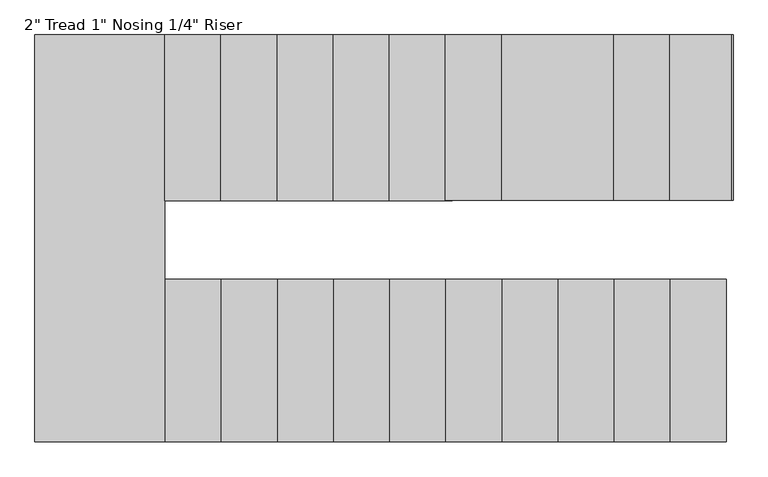
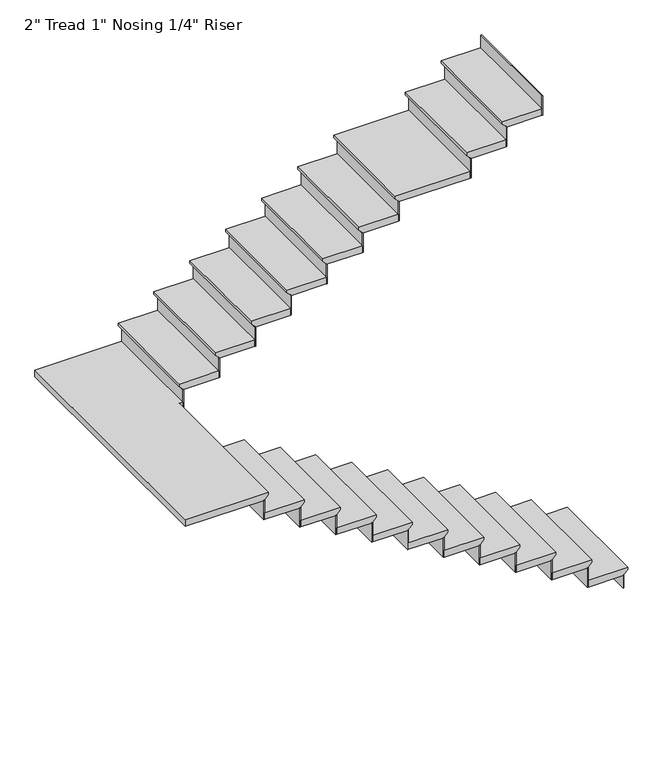
"""IFC4 building model written with IfcOpenShell, lengths in millimetres: stair flight geometry."""

from ifc_helpers import new_model, si_unit, origin, place, context, project, spatial, faceted_brep, source, transform, mapped, element, save


def stair_flight_d547b7c1(model_context):
    return source(origin(), model_context, "Body", "Brep", [
        faceted_brep([(-3117.2664982, -7431.6600272, 6222.0928571), (-3117.2664982, -7431.6600272, 6241.1428571), (-3117.2664982, -8168.2600272, 6241.1428571), (-3117.2664982, -8168.2600272, 6222.0928571), (-3142.6664982, -7431.6600272, 6196.6928571), (-3142.6664982, -8168.2600272, 6196.6928571), (-3396.6664982, -7431.6600272, 6241.1428571), (-3396.6664982, -8168.2600272, 6241.1428571), (-3142.6664982, -8168.2600272, 6190.3428571), (-3396.6664982, -8168.2600272, 6190.3428571), (-3396.6664982, -7431.6600272, 6190.3428571), (-3142.6664982, -7431.6600272, 6190.3428571)], [[[0, 1, 2, 3]], [[4, 0, 3, 5]], [[2, 1, 6, 7]], [[8, 9, 10, 11]], [[2, 7, 9, 8, 5, 3]], [[8, 11, 4, 5]], [[6, 1, 0, 4, 11, 10]], [[7, 6, 10, 9]]]),
        faceted_brep([(-3142.6664982, -7431.6600272, 6190.3428571), (-3142.6664982, -7431.6600272, 6096.0), (-3149.0164982, -7431.6600272, 6096.0), (-3149.0164982, -7431.6600272, 6190.3428571), (-3142.6664982, -8168.2600272, 6190.3428571), (-3149.0164982, -8168.2600272, 6190.3428571), (-3149.0164982, -8168.2600272, 6096.0), (-3142.6664982, -8168.2600272, 6096.0)], [[[0, 1, 2, 3]], [[4, 5, 6, 7]], [[1, 0, 4, 7]], [[2, 1, 7, 6]], [[3, 2, 6, 5]], [[0, 3, 5, 4]]]),
        faceted_brep([(-3396.6664982, -7431.6600272, 6335.4857143), (-3396.6664982, -7431.6600272, 6190.3428571), (-3403.0164982, -7431.6600272, 6190.3428571), (-3403.0164982, -7431.6600272, 6335.4857143), (-3396.6664982, -8168.2600272, 6335.4857143), (-3403.0164982, -8168.2600272, 6335.4857143), (-3403.0164982, -8168.2600272, 6190.3428571), (-3396.6664982, -8168.2600272, 6190.3428571)], [[[0, 1, 2, 3]], [[4, 5, 6, 7]], [[1, 0, 4, 7]], [[2, 1, 7, 6]], [[3, 2, 6, 5]], [[0, 3, 5, 4]]]),
        faceted_brep([(-3371.2664982, -8168.2600272, 6386.2857143), (-3371.2664982, -7431.6600272, 6386.2857143), (-3650.6664982, -7431.6600272, 6386.2857143), (-3650.6664982, -8168.2600272, 6386.2857143), (-3396.6664982, -8168.2600272, 6335.4857143), (-3650.6664982, -8168.2600272, 6335.4857143), (-3650.6664982, -7431.6600272, 6335.4857143), (-3396.6664982, -7431.6600272, 6335.4857143), (-3396.6664982, -8168.2600272, 6341.8357143), (-3371.2664982, -8168.2600272, 6367.2357143), (-3396.6664982, -7431.6600272, 6341.8357143), (-3371.2664982, -7431.6600272, 6367.2357143)], [[[0, 1, 2, 3]], [[4, 5, 6, 7]], [[0, 3, 5, 4, 8, 9]], [[4, 7, 10, 8]], [[2, 1, 11, 10, 7, 6]], [[3, 2, 6, 5]], [[11, 1, 0, 9]], [[10, 11, 9, 8]]]),
        faceted_brep([(-3650.6664982, -7431.6600272, 6480.6285714), (-3650.6664982, -7431.6600272, 6335.4857143), (-3657.0164982, -7431.6600272, 6335.4857143), (-3657.0164982, -7431.6600272, 6480.6285714), (-3650.6664982, -8168.2600272, 6480.6285714), (-3657.0164982, -8168.2600272, 6480.6285714), (-3657.0164982, -8168.2600272, 6335.4857143), (-3650.6664982, -8168.2600272, 6335.4857143)], [[[0, 1, 2, 3]], [[4, 5, 6, 7]], [[1, 0, 4, 7]], [[2, 1, 7, 6]], [[3, 2, 6, 5]], [[0, 3, 5, 4]]]),
        faceted_brep([(-3625.2664982, -8168.2600272, 6531.4285714), (-3625.2664982, -7431.6600272, 6531.4285714), (-3904.6664982, -7431.6600272, 6531.4285714), (-3904.6664982, -8168.2600272, 6531.4285714), (-3650.6664982, -8168.2600272, 6480.6285714), (-3904.6664982, -8168.2600272, 6480.6285714), (-3904.6664982, -7431.6600272, 6480.6285714), (-3650.6664982, -7431.6600272, 6480.6285714), (-3650.6664982, -8168.2600272, 6486.9785714), (-3625.2664982, -8168.2600272, 6512.3785714), (-3650.6664982, -7431.6600272, 6486.9785714), (-3625.2664982, -7431.6600272, 6512.3785714)], [[[0, 1, 2, 3]], [[4, 5, 6, 7]], [[0, 3, 5, 4, 8, 9]], [[4, 7, 10, 8]], [[2, 1, 11, 10, 7, 6]], [[3, 2, 6, 5]], [[11, 1, 0, 9]], [[10, 11, 9, 8]]]),
        faceted_brep([(-3904.6664982, -7431.6600272, 6625.7714286), (-3904.6664982, -7431.6600272, 6480.6285714), (-3911.0164982, -7431.6600272, 6480.6285714), (-3911.0164982, -7431.6600272, 6625.7714286), (-3904.6664982, -8168.2600272, 6625.7714286), (-3911.0164982, -8168.2600272, 6625.7714286), (-3911.0164982, -8168.2600272, 6480.6285714), (-3904.6664982, -8168.2600272, 6480.6285714)], [[[0, 1, 2, 3]], [[4, 5, 6, 7]], [[1, 0, 4, 7]], [[2, 1, 7, 6]], [[3, 2, 6, 5]], [[0, 3, 5, 4]]]),
        faceted_brep([(-3879.2664982, -8168.2600272, 6676.5714286), (-3879.2664982, -7431.6600272, 6676.5714286), (-4158.6664982, -7431.6600272, 6676.5714286), (-4158.6664982, -8168.2600272, 6676.5714286), (-3904.6664982, -8168.2600272, 6625.7714286), (-4158.6664982, -8168.2600272, 6625.7714286), (-4158.6664982, -7431.6600272, 6625.7714286), (-3904.6664982, -7431.6600272, 6625.7714286), (-3904.6664982, -8168.2600272, 6632.1214286), (-3879.2664982, -8168.2600272, 6657.5214286), (-3904.6664982, -7431.6600272, 6632.1214286), (-3879.2664982, -7431.6600272, 6657.5214286)], [[[0, 1, 2, 3]], [[4, 5, 6, 7]], [[0, 3, 5, 4, 8, 9]], [[4, 7, 10, 8]], [[2, 1, 11, 10, 7, 6]], [[3, 2, 6, 5]], [[11, 1, 0, 9]], [[10, 11, 9, 8]]]),
        faceted_brep([(-4158.6664982, -7431.6600272, 6770.9142857), (-4158.6664982, -7431.6600272, 6625.7714286), (-4165.0164982, -7431.6600272, 6625.7714286), (-4165.0164982, -7431.6600272, 6770.9142857), (-4158.6664982, -8168.2600272, 6770.9142857), (-4165.0164982, -8168.2600272, 6770.9142857), (-4165.0164982, -8168.2600272, 6625.7714286), (-4158.6664982, -8168.2600272, 6625.7714286)], [[[0, 1, 2, 3]], [[4, 5, 6, 7]], [[1, 0, 4, 7]], [[2, 1, 7, 6]], [[3, 2, 6, 5]], [[0, 3, 5, 4]]]),
        faceted_brep([(-4133.2664982, -8168.2600272, 6821.7142857), (-4133.2664982, -7431.6600272, 6821.7142857), (-4412.6664982, -7431.6600272, 6821.7142857), (-4412.6664982, -8168.2600272, 6821.7142857), (-4158.6664982, -8168.2600272, 6770.9142857), (-4412.6664982, -8168.2600272, 6770.9142857), (-4412.6664982, -7431.6600272, 6770.9142857), (-4158.6664982, -7431.6600272, 6770.9142857), (-4158.6664982, -8168.2600272, 6777.2642857), (-4133.2664982, -8168.2600272, 6802.6642857), (-4158.6664982, -7431.6600272, 6777.2642857), (-4133.2664982, -7431.6600272, 6802.6642857)], [[[0, 1, 2, 3]], [[4, 5, 6, 7]], [[0, 3, 5, 4, 8, 9]], [[4, 7, 10, 8]], [[2, 1, 11, 10, 7, 6]], [[3, 2, 6, 5]], [[11, 1, 0, 9]], [[10, 11, 9, 8]]]),
        faceted_brep([(-4412.6664982, -7431.6600272, 6916.0571429), (-4412.6664982, -7431.6600272, 6770.9142857), (-4419.0164982, -7431.6600272, 6770.9142857), (-4419.0164982, -7431.6600272, 6916.0571429), (-4412.6664982, -8168.2600272, 6916.0571429), (-4419.0164982, -8168.2600272, 6916.0571429), (-4419.0164982, -8168.2600272, 6770.9142857), (-4412.6664982, -8168.2600272, 6770.9142857)], [[[0, 1, 2, 3]], [[4, 5, 6, 7]], [[1, 0, 4, 7]], [[2, 1, 7, 6]], [[3, 2, 6, 5]], [[0, 3, 5, 4]]]),
        faceted_brep([(-4387.2664982, -8168.2600272, 6966.8571429), (-4387.2664982, -7431.6600272, 6966.8571429), (-4666.6664982, -7431.6600272, 6966.8571429), (-4666.6664982, -8168.2600272, 6966.8571429), (-4412.6664982, -8168.2600272, 6916.0571429), (-4666.6664982, -8168.2600272, 6916.0571429), (-4666.6664982, -7431.6600272, 6916.0571429), (-4412.6664982, -7431.6600272, 6916.0571429), (-4412.6664982, -8168.2600272, 6922.4071429), (-4387.2664982, -8168.2600272, 6947.8071429), (-4412.6664982, -7431.6600272, 6922.4071429), (-4387.2664982, -7431.6600272, 6947.8071429)], [[[0, 1, 2, 3]], [[4, 5, 6, 7]], [[0, 3, 5, 4, 8, 9]], [[4, 7, 10, 8]], [[2, 1, 11, 10, 7, 6]], [[3, 2, 6, 5]], [[11, 1, 0, 9]], [[10, 11, 9, 8]]]),
        faceted_brep([(-4666.6664982, -7431.6600272, 7061.2), (-4666.6664982, -7431.6600272, 6916.0571429), (-4673.0164982, -7431.6600272, 6916.0571429), (-4673.0164982, -7431.6600272, 7061.2), (-4666.6664982, -8168.2600272, 7061.2), (-4673.0164982, -8168.2600272, 7061.2), (-4673.0164982, -8168.2600272, 6916.0571429), (-4666.6664982, -8168.2600272, 6916.0571429)], [[[0, 1, 2, 3]], [[4, 5, 6, 7]], [[1, 0, 4, 7]], [[2, 1, 7, 6]], [[3, 2, 6, 5]], [[0, 3, 5, 4]]]),
        faceted_brep([(-4641.2664982, -8168.2600272, 7112.0), (-4641.2664982, -7431.6600272, 7112.0), (-4920.6664982, -7431.6600272, 7112.0), (-4920.6664982, -8168.2600272, 7112.0), (-4666.6664982, -8168.2600272, 7061.2), (-4920.6664982, -8168.2600272, 7061.2), (-4920.6664982, -7431.6600272, 7061.2), (-4666.6664982, -7431.6600272, 7061.2), (-4666.6664982, -8168.2600272, 7067.55), (-4641.2664982, -8168.2600272, 7092.95), (-4666.6664982, -7431.6600272, 7067.55), (-4641.2664982, -7431.6600272, 7092.95)], [[[0, 1, 2, 3]], [[4, 5, 6, 7]], [[0, 3, 5, 4, 8, 9]], [[4, 7, 10, 8]], [[2, 1, 11, 10, 7, 6]], [[3, 2, 6, 5]], [[11, 1, 0, 9]], [[10, 11, 9, 8]]]),
        faceted_brep([(-4920.6664982, -7431.6600272, 7206.3428571), (-4920.6664982, -7431.6600272, 7061.2), (-4927.0164982, -7431.6600272, 7061.2), (-4927.0164982, -7431.6600272, 7206.3428571), (-4920.6664982, -8168.2600272, 7206.3428571), (-4927.0164982, -8168.2600272, 7206.3428571), (-4927.0164982, -8168.2600272, 7061.2), (-4920.6664982, -8168.2600272, 7061.2)], [[[0, 1, 2, 3]], [[4, 5, 6, 7]], [[1, 0, 4, 7]], [[2, 1, 7, 6]], [[3, 2, 6, 5]], [[0, 3, 5, 4]]]),
        faceted_brep([(-4895.2664982, -8168.2600272, 7257.1428571), (-4895.2664982, -7431.6600272, 7257.1428571), (-5174.6664982, -7431.6600272, 7257.1428571), (-5174.6664982, -8168.2600272, 7257.1428571), (-4920.6664982, -8168.2600272, 7206.3428571), (-5174.6664982, -8168.2600272, 7206.3428571), (-5174.6664982, -7431.6600272, 7206.3428571), (-4920.6664982, -7431.6600272, 7206.3428571), (-4920.6664982, -8168.2600272, 7212.6928571), (-4895.2664982, -8168.2600272, 7238.0928571), (-4920.6664982, -7431.6600272, 7212.6928571), (-4895.2664982, -7431.6600272, 7238.0928571)], [[[0, 1, 2, 3]], [[4, 5, 6, 7]], [[0, 3, 5, 4, 8, 9]], [[4, 7, 10, 8]], [[2, 1, 11, 10, 7, 6]], [[3, 2, 6, 5]], [[11, 1, 0, 9]], [[10, 11, 9, 8]]]),
        faceted_brep([(-5174.6664982, -7431.6600272, 7351.4857143), (-5174.6664982, -7431.6600272, 7206.3428571), (-5181.0164982, -7431.6600272, 7206.3428571), (-5181.0164982, -7431.6600272, 7351.4857143), (-5174.6664982, -8168.2600272, 7351.4857143), (-5181.0164982, -8168.2600272, 7351.4857143), (-5181.0164982, -8168.2600272, 7206.3428571), (-5174.6664982, -8168.2600272, 7206.3428571)], [[[0, 1, 2, 3]], [[4, 5, 6, 7]], [[1, 0, 4, 7]], [[2, 1, 7, 6]], [[3, 2, 6, 5]], [[0, 3, 5, 4]]]),
        faceted_brep([(-5149.2664982, -8168.2600272, 7402.2857143), (-5149.2664982, -7431.6600272, 7402.2857143), (-5428.6664982, -7431.6600272, 7402.2857143), (-5428.6664982, -8168.2600272, 7402.2857143), (-5174.6664982, -8168.2600272, 7351.4857143), (-5428.6664982, -8168.2600272, 7351.4857143), (-5428.6664982, -7431.6600272, 7351.4857143), (-5174.6664982, -7431.6600272, 7351.4857143), (-5174.6664982, -8168.2600272, 7357.8357143), (-5149.2664982, -8168.2600272, 7383.2357143), (-5174.6664982, -7431.6600272, 7357.8357143), (-5149.2664982, -7431.6600272, 7383.2357143)], [[[0, 1, 2, 3]], [[4, 5, 6, 7]], [[0, 3, 5, 4, 8, 9]], [[4, 7, 10, 8]], [[2, 1, 11, 10, 7, 6]], [[3, 2, 6, 5]], [[11, 1, 0, 9]], [[10, 11, 9, 8]]]),
        faceted_brep([(-5428.6664982, -7431.6600272, 7496.6285714), (-5428.6664982, -7431.6600272, 7351.4857143), (-5435.0164982, -7431.6600272, 7351.4857143), (-5435.0164982, -7431.6600272, 7496.6285714), (-5428.6664982, -8168.2600272, 7496.6285714), (-5435.0164982, -8168.2600272, 7496.6285714), (-5435.0164982, -8168.2600272, 7351.4857143), (-5428.6664982, -8168.2600272, 7351.4857143)], [[[0, 1, 2, 3]], [[4, 5, 6, 7]], [[1, 0, 4, 7]], [[2, 1, 7, 6]], [[3, 2, 6, 5]], [[0, 3, 5, 4]]]),
        faceted_brep([(-5403.2664982, -8168.2600272, 7547.4285714), (-5403.2664982, -7431.6600272, 7547.4285714), (-5682.6664982, -7431.6600272, 7547.4285714), (-5682.6664982, -8168.2600272, 7547.4285714), (-5428.6664982, -8168.2600272, 7496.6285714), (-5682.6664982, -8168.2600272, 7496.6285714), (-5682.6664982, -7431.6600272, 7496.6285714), (-5428.6664982, -7431.6600272, 7496.6285714), (-5428.6664982, -8168.2600272, 7502.9785714), (-5403.2664982, -8168.2600272, 7528.3785714), (-5428.6664982, -7431.6600272, 7502.9785714), (-5403.2664982, -7431.6600272, 7528.3785714)], [[[0, 1, 2, 3]], [[4, 5, 6, 7]], [[0, 3, 5, 4, 8, 9]], [[4, 7, 10, 8]], [[2, 1, 11, 10, 7, 6]], [[3, 2, 6, 5]], [[11, 1, 0, 9]], [[10, 11, 9, 8]]]),
        faceted_brep([(-5682.6664982, -7431.6600272, 7641.7714286), (-5682.6664982, -7431.6600272, 7496.6285714), (-5689.0164982, -7431.6600272, 7496.6285714), (-5689.0164982, -7431.6600272, 7641.7714286), (-5682.6664982, -8168.2600272, 7641.7714286), (-5689.0164982, -8168.2600272, 7641.7714286), (-5689.0164982, -8168.2600272, 7496.6285714), (-5682.6664982, -8168.2600272, 7496.6285714)], [[[0, 1, 2, 3]], [[4, 5, 6, 7]], [[1, 0, 4, 7]], [[2, 1, 7, 6]], [[3, 2, 6, 5]], [[0, 3, 5, 4]]]),
        faceted_brep([(-5631.8664982, -6326.7600272, 7692.5714286), (-6245.2108866, -6326.7600272, 7692.5714286), (-6245.2108866, -8168.2600272, 7692.5714286), (-5657.2664982, -8168.2600272, 7692.5714286), (-5657.2664982, -7076.0600272, 7692.5714286), (-5631.8664982, -7076.0600272, 7692.5714286), (-6245.2108866, -6326.7600272, 7641.7714286), (-5631.8664982, -6326.7600272, 7641.7714286), (-5631.8664982, -7076.0600272, 7641.7714286), (-5657.2664982, -7076.0600272, 7641.7714286), (-5657.2664982, -7431.6600272, 7641.7714286), (-5682.6664982, -7431.6600272, 7641.7714286), (-5682.6664982, -8168.2600272, 7641.7714286), (-6245.2108866, -8168.2600272, 7641.7714286), (-5682.6664982, -8168.2600272, 7648.1214286), (-5657.2664982, -8168.2600272, 7673.5214286), (-5682.6664982, -7431.6600272, 7648.1214286), (-5657.2664982, -7431.6600272, 7673.5214286)], [[[0, 1, 2, 3, 4, 5]], [[6, 7, 8, 9, 10, 11, 12, 13]], [[1, 0, 7, 6]], [[2, 1, 6, 13]], [[3, 2, 13, 12, 14, 15]], [[12, 11, 16, 14]], [[11, 10, 17, 16]], [[4, 3, 15, 17, 10, 9]], [[5, 4, 9, 8]], [[0, 5, 8, 7]], [[15, 14, 16, 17]]]),
        faceted_brep([(-5631.8664982, -7076.0600272, 7786.9142857), (-5631.8664982, -7076.0600272, 7641.7714286), (-5625.5164982, -7076.0600272, 7641.7714286), (-5625.5164982, -7076.0600272, 7786.9142857), (-5631.8664982, -6326.7600272, 7786.9142857), (-5625.5164982, -6326.7600272, 7786.9142857), (-5625.5164982, -6326.7600272, 7641.7714286), (-5631.8664982, -6326.7600272, 7641.7714286)], [[[0, 1, 2, 3]], [[4, 5, 6, 7]], [[1, 0, 4, 7]], [[2, 1, 7, 6]], [[3, 2, 6, 5]], [[0, 3, 5, 4]]]),
        faceted_brep([(-5657.2664982, -6326.7600272, 7837.7142857), (-5657.2664982, -7076.0600272, 7837.7142857), (-5377.8664982, -7076.0600272, 7837.7142857), (-5377.8664982, -6326.7600272, 7837.7142857), (-5631.8664982, -6326.7600272, 7786.9142857), (-5377.8664982, -6326.7600272, 7786.9142857), (-5377.8664982, -7076.0600272, 7786.9142857), (-5631.8664982, -7076.0600272, 7786.9142857), (-5631.8664982, -6326.7600272, 7793.2642857), (-5657.2664982, -6326.7600272, 7818.6642857), (-5631.8664982, -7076.0600272, 7793.2642857), (-5657.2664982, -7076.0600272, 7818.6642857)], [[[0, 1, 2, 3]], [[4, 5, 6, 7]], [[0, 3, 5, 4, 8, 9]], [[4, 7, 10, 8]], [[2, 1, 11, 10, 7, 6]], [[3, 2, 6, 5]], [[11, 1, 0, 9]], [[10, 11, 9, 8]]]),
        faceted_brep([(-5377.8664982, -7076.0600272, 7932.0571429), (-5377.8664982, -7076.0600272, 7786.9142857), (-5371.5164982, -7076.0600272, 7786.9142857), (-5371.5164982, -7076.0600272, 7932.0571429), (-5377.8664982, -6326.7600272, 7932.0571429), (-5371.5164982, -6326.7600272, 7932.0571429), (-5371.5164982, -6326.7600272, 7786.9142857), (-5377.8664982, -6326.7600272, 7786.9142857)], [[[0, 1, 2, 3]], [[4, 5, 6, 7]], [[1, 0, 4, 7]], [[2, 1, 7, 6]], [[3, 2, 6, 5]], [[0, 3, 5, 4]]]),
        faceted_brep([(-5403.2664982, -6326.7600272, 7982.8571429), (-5403.2664982, -7076.0600272, 7982.8571429), (-5123.8664982, -7076.0600272, 7982.8571429), (-5123.8664982, -6326.7600272, 7982.8571429), (-5377.8664982, -6326.7600272, 7932.0571429), (-5123.8664982, -6326.7600272, 7932.0571429), (-5123.8664982, -7076.0600272, 7932.0571429), (-5377.8664982, -7076.0600272, 7932.0571429), (-5377.8664982, -6326.7600272, 7938.4071429), (-5403.2664982, -6326.7600272, 7963.8071429), (-5377.8664982, -7076.0600272, 7938.4071429), (-5403.2664982, -7076.0600272, 7963.8071429)], [[[0, 1, 2, 3]], [[4, 5, 6, 7]], [[0, 3, 5, 4, 8, 9]], [[4, 7, 10, 8]], [[2, 1, 11, 10, 7, 6]], [[3, 2, 6, 5]], [[11, 1, 0, 9]], [[10, 11, 9, 8]]]),
        faceted_brep([(-5123.8664982, -7076.0600272, 8077.2), (-5123.8664982, -7076.0600272, 7932.0571429), (-5117.5164982, -7076.0600272, 7932.0571429), (-5117.5164982, -7076.0600272, 8077.2), (-5123.8664982, -6326.7600272, 8077.2), (-5117.5164982, -6326.7600272, 8077.2), (-5117.5164982, -6326.7600272, 7932.0571429), (-5123.8664982, -6326.7600272, 7932.0571429)], [[[0, 1, 2, 3]], [[4, 5, 6, 7]], [[1, 0, 4, 7]], [[2, 1, 7, 6]], [[3, 2, 6, 5]], [[0, 3, 5, 4]]]),
        faceted_brep([(-5149.2664982, -6326.7600272, 8128.0), (-5149.2664982, -7076.0600272, 8128.0), (-4869.8664982, -7076.0600272, 8128.0), (-4869.8664982, -6326.7600272, 8128.0), (-5123.8664982, -6326.7600272, 8077.2), (-4869.8664982, -6326.7600272, 8077.2), (-4869.8664982, -7076.0600272, 8077.2), (-5123.8664982, -7076.0600272, 8077.2), (-5123.8664982, -6326.7600272, 8083.55), (-5149.2664982, -6326.7600272, 8108.95), (-5123.8664982, -7076.0600272, 8083.55), (-5149.2664982, -7076.0600272, 8108.95)], [[[0, 1, 2, 3]], [[4, 5, 6, 7]], [[0, 3, 5, 4, 8, 9]], [[4, 7, 10, 8]], [[2, 1, 11, 10, 7, 6]], [[3, 2, 6, 5]], [[11, 1, 0, 9]], [[10, 11, 9, 8]]]),
        faceted_brep([(-4869.8664982, -7076.0600272, 8222.3428571), (-4869.8664982, -7076.0600272, 8077.2), (-4863.5164982, -7076.0600272, 8077.2), (-4863.5164982, -7076.0600272, 8222.3428571), (-4869.8664982, -6326.7600272, 8222.3428571), (-4863.5164982, -6326.7600272, 8222.3428571), (-4863.5164982, -6326.7600272, 8077.2), (-4869.8664982, -6326.7600272, 8077.2)], [[[0, 1, 2, 3]], [[4, 5, 6, 7]], [[1, 0, 4, 7]], [[2, 1, 7, 6]], [[3, 2, 6, 5]], [[0, 3, 5, 4]]]),
        faceted_brep([(-4895.2664982, -6326.7600272, 8273.1428571), (-4895.2664982, -7076.0600272, 8273.1428571), (-4615.8664982, -7076.0600272, 8273.1428571), (-4615.8664982, -6326.7600272, 8273.1428571), (-4869.8664982, -6326.7600272, 8222.3428571), (-4615.8664982, -6326.7600272, 8222.3428571), (-4615.8664982, -7076.0600272, 8222.3428571), (-4869.8664982, -7076.0600272, 8222.3428571), (-4869.8664982, -6326.7600272, 8228.6928571), (-4895.2664982, -6326.7600272, 8254.0928571), (-4869.8664982, -7076.0600272, 8228.6928571), (-4895.2664982, -7076.0600272, 8254.0928571)], [[[0, 1, 2, 3]], [[4, 5, 6, 7]], [[0, 3, 5, 4, 8, 9]], [[4, 7, 10, 8]], [[2, 1, 11, 10, 7, 6]], [[3, 2, 6, 5]], [[11, 1, 0, 9]], [[10, 11, 9, 8]]]),
        faceted_brep([(-4615.8664982, -7076.0600272, 8367.4857143), (-4615.8664982, -7076.0600272, 8222.3428571), (-4609.5164982, -7076.0600272, 8222.3428571), (-4609.5164982, -7076.0600272, 8367.4857143), (-4615.8664982, -6326.7600272, 8367.4857143), (-4609.5164982, -6326.7600272, 8367.4857143), (-4609.5164982, -6326.7600272, 8222.3428571), (-4615.8664982, -6326.7600272, 8222.3428571)], [[[0, 1, 2, 3]], [[4, 5, 6, 7]], [[1, 0, 4, 7]], [[2, 1, 7, 6]], [[3, 2, 6, 5]], [[0, 3, 5, 4]]]),
        faceted_brep([(-4641.2664982, -6326.7600272, 8418.2857143), (-4641.2664982, -7076.0600272, 8418.2857143), (-4361.8664982, -7076.0600272, 8418.2857143), (-4361.8664982, -6326.7600272, 8418.2857143), (-4615.8664982, -6326.7600272, 8367.4857143), (-4361.8664982, -6326.7600272, 8367.4857143), (-4361.8664982, -7076.0600272, 8367.4857143), (-4615.8664982, -7076.0600272, 8367.4857143), (-4615.8664982, -6326.7600272, 8373.8357143), (-4641.2664982, -6326.7600272, 8399.2357143), (-4615.8664982, -7076.0600272, 8373.8357143), (-4641.2664982, -7076.0600272, 8399.2357143)], [[[0, 1, 2, 3]], [[4, 5, 6, 7]], [[0, 3, 5, 4, 8, 9]], [[4, 7, 10, 8]], [[2, 1, 11, 10, 7, 6]], [[3, 2, 6, 5]], [[11, 1, 0, 9]], [[10, 11, 9, 8]]]),
        faceted_brep([(-4361.8664982, -7076.0600272, 8512.6285714), (-4361.8664982, -7076.0600272, 8367.4857143), (-4355.5164982, -7076.0600272, 8367.4857143), (-4355.5164982, -7076.0600272, 8512.6285714), (-4361.8664982, -6326.7600272, 8512.6285714), (-4355.5164982, -6326.7600272, 8512.6285714), (-4355.5164982, -6326.7600272, 8367.4857143), (-4361.8664982, -6326.7600272, 8367.4857143)], [[[0, 1, 2, 3]], [[4, 5, 6, 7]], [[1, 0, 4, 7]], [[2, 1, 7, 6]], [[3, 2, 6, 5]], [[0, 3, 5, 4]]]),
        faceted_brep([(-4387.2664982, -6326.7600272, 8563.4285714), (-4387.2664982, -7076.0600272, 8563.4285714), (-4107.8664982, -7076.0600272, 8563.4285714), (-4107.8664982, -6326.7600272, 8563.4285714), (-4361.8664982, -6326.7600272, 8512.6285714), (-4107.8664982, -6326.7600272, 8512.6285714), (-4107.8664982, -7076.0600272, 8512.6285714), (-4361.8664982, -7076.0600272, 8512.6285714), (-4361.8664982, -6326.7600272, 8518.9785714), (-4387.2664982, -6326.7600272, 8544.3785714), (-4361.8664982, -7076.0600272, 8518.9785714), (-4387.2664982, -7076.0600272, 8544.3785714)], [[[0, 1, 2, 3]], [[4, 5, 6, 7]], [[0, 3, 5, 4, 8, 9]], [[4, 7, 10, 8]], [[2, 1, 11, 10, 7, 6]], [[3, 2, 6, 5]], [[11, 1, 0, 9]], [[10, 11, 9, 8]]]),
        faceted_brep([(-4107.8664982, -7076.0600272, 8657.7714286), (-4107.8664982, -7076.0600272, 8512.6285714), (-4101.5164982, -7076.0600272, 8512.6285714), (-4101.5164982, -7076.0600272, 8657.7714286), (-4107.8664982, -6326.7600272, 8657.7714286), (-4101.5164982, -6326.7600272, 8657.7714286), (-4101.5164982, -6326.7600272, 8512.6285714), (-4107.8664982, -6326.7600272, 8512.6285714)], [[[0, 1, 2, 3]], [[4, 5, 6, 7]], [[1, 0, 4, 7]], [[2, 1, 7, 6]], [[3, 2, 6, 5]], [[0, 3, 5, 4]]]),
        faceted_brep([(-4133.2664982, -6326.7600272, 8708.5714286), (-4133.2664982, -7076.0600272, 8708.5714286), (-3599.8664982, -7076.0600272, 8708.5714286), (-3599.8664982, -6326.7600272, 8708.5714286), (-4107.8664982, -6326.7600272, 8657.7714286), (-3599.8664982, -6326.7600272, 8657.7714286), (-3599.8664982, -7076.0600272, 8657.7714286), (-4107.8664982, -7076.0600272, 8657.7714286), (-4107.8664982, -6326.7600272, 8664.1214286), (-4133.2664982, -6326.7600272, 8689.5214286), (-4107.8664982, -7076.0600272, 8664.1214286), (-4133.2664982, -7076.0600272, 8689.5214286)], [[[0, 1, 2, 3]], [[4, 5, 6, 7]], [[0, 3, 5, 4, 8, 9]], [[4, 7, 10, 8]], [[2, 1, 11, 10, 7, 6]], [[3, 2, 6, 5]], [[11, 1, 0, 9]], [[10, 11, 9, 8]]]),
        faceted_brep([(-3599.8664982, -7076.0600272, 8802.9142857), (-3599.8664982, -7076.0600272, 8657.7714286), (-3593.5164982, -7076.0600272, 8657.7714286), (-3593.5164982, -7076.0600272, 8802.9142857), (-3599.8664982, -6326.7600272, 8802.9142857), (-3593.5164982, -6326.7600272, 8802.9142857), (-3593.5164982, -6326.7600272, 8657.7714286), (-3599.8664982, -6326.7600272, 8657.7714286)], [[[0, 1, 2, 3]], [[4, 5, 6, 7]], [[1, 0, 4, 7]], [[2, 1, 7, 6]], [[3, 2, 6, 5]], [[0, 3, 5, 4]]]),
        faceted_brep([(-3625.2664982, -6326.7600272, 8853.7142857), (-3625.2664982, -7076.0600272, 8853.7142857), (-3345.8664982, -7076.0600272, 8853.7142857), (-3345.8664982, -6326.7600272, 8853.7142857), (-3599.8664982, -6326.7600272, 8802.9142857), (-3345.8664982, -6326.7600272, 8802.9142857), (-3345.8664982, -7076.0600272, 8802.9142857), (-3599.8664982, -7076.0600272, 8802.9142857), (-3599.8664982, -6326.7600272, 8809.2642857), (-3625.2664982, -6326.7600272, 8834.6642857), (-3599.8664982, -7076.0600272, 8809.2642857), (-3625.2664982, -7076.0600272, 8834.6642857)], [[[0, 1, 2, 3]], [[4, 5, 6, 7]], [[0, 3, 5, 4, 8, 9]], [[4, 7, 10, 8]], [[2, 1, 11, 10, 7, 6]], [[3, 2, 6, 5]], [[11, 1, 0, 9]], [[10, 11, 9, 8]]]),
        faceted_brep([(-3345.8664982, -7076.0600272, 8948.0571429), (-3345.8664982, -7076.0600272, 8802.9142857), (-3339.5164982, -7076.0600272, 8802.9142857), (-3339.5164982, -7076.0600272, 8948.0571429), (-3345.8664982, -6326.7600272, 8948.0571429), (-3339.5164982, -6326.7600272, 8948.0571429), (-3339.5164982, -6326.7600272, 8802.9142857), (-3345.8664982, -6326.7600272, 8802.9142857)], [[[0, 1, 2, 3]], [[4, 5, 6, 7]], [[1, 0, 4, 7]], [[2, 1, 7, 6]], [[3, 2, 6, 5]], [[0, 3, 5, 4]]]),
        faceted_brep([(-3091.8664982, -7076.0600272, 9093.2), (-3091.8664982, -7076.0600272, 8948.0571429), (-3085.5164982, -7076.0600272, 8948.0571429), (-3085.5164982, -7076.0600272, 9093.2), (-3091.8664982, -6326.7600272, 9093.2), (-3085.5164982, -6326.7600272, 9093.2), (-3085.5164982, -6326.7600272, 8948.0571429), (-3091.8664982, -6326.7600272, 8948.0571429)], [[[0, 1, 2, 3]], [[4, 5, 6, 7]], [[1, 0, 4, 7]], [[2, 1, 7, 6]], [[3, 2, 6, 5]], [[0, 3, 5, 4]]]),
        faceted_brep([(-3371.2664982, -6326.7600272, 8998.8571429), (-3371.2664982, -7076.0600272, 8998.8571429), (-3091.8664982, -7076.0600272, 8998.8571429), (-3091.8664982, -6326.7600272, 8998.8571429), (-3345.8664982, -6326.7600272, 8948.0571429), (-3091.8664982, -6326.7600272, 8948.0571429), (-3091.8664982, -7076.0600272, 8948.0571429), (-3345.8664982, -7076.0600272, 8948.0571429), (-3345.8664982, -6326.7600272, 8954.4071429), (-3371.2664982, -6326.7600272, 8979.8071429), (-3345.8664982, -7076.0600272, 8954.4071429), (-3371.2664982, -7076.0600272, 8979.8071429)], [[[0, 1, 2, 3]], [[4, 5, 6, 7]], [[0, 3, 5, 4, 8, 9]], [[4, 7, 10, 8]], [[2, 1, 11, 10, 7, 6]], [[3, 2, 6, 5]], [[11, 1, 0, 9]], [[10, 11, 9, 8]]]),
    ])


if __name__ == "__main__":
    model = new_model("IFC4")
    model_context = context("Model", 3, world=origin())
    ifc_project = project(units=[si_unit("LENGTHUNIT", "METRE", prefix="MILLI")], contexts=[model_context])
    site = spatial("IfcSite", under=ifc_project)
    building = spatial("IfcBuilding", under=site)
    placement = place(None, origin())
    stair_flight_shape = stair_flight_d547b7c1(model_context)
    element("IfcStairFlight", 1, ObjectType="2\" Tread 1\" Nosing 1/4\" Riser", at=placement, inside=building, context=model_context, shape_type="MappedRepresentation", body=[
        mapped(stair_flight_shape, transform((0.0, 0.0, 0.0), x_axis=(1.0, 0.0, 0.0), y_axis=(0.0, 1.0, 0.0), z_axis=(0.0, 0.0, 1.0))),
    ])
    save(model, "model.ifc")
